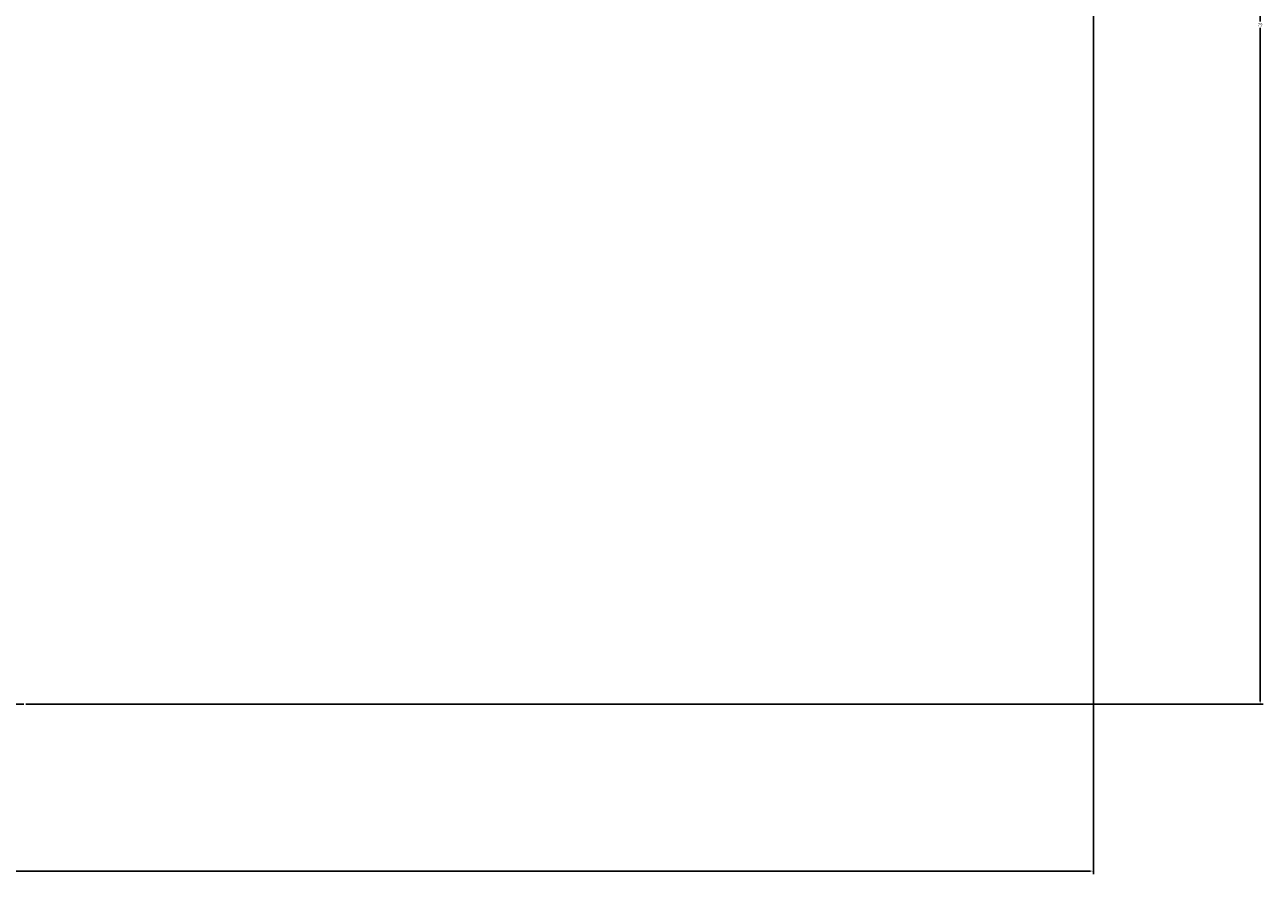
# Model space of a CAD drawing. Units: millimetres. Extents: x -136 to 10, y 158 to 257.
# Tile 4 of 6: x -62 to 10, y 158 to 208. Entities that reach past the tile are written whole.
import ezdxf

# ---------------------------------------------------------------- set-up
doc = ezdxf.new("R2010")
doc.units = ezdxf.units.MM
doc.layers.add('M-DIMS', color=2, linetype='Continuous', lineweight=18)
doc.styles.get("Standard").update_dxf_attribs({"font": 'arial.ttf'})
doc.dimstyles.get("Standard").update_dxf_attribs({"dimtxt": 0.18, "dimasz": 0.18, "dimexe": 0.18, "dimexo": 0.0625, "dimgap": 0.09, "dimtad": 0, "dimtih": 1, "dimtoh": 1, "dimdec": 4, "dimzin": 0, "dimdsep": 46, "dimtxsty": 'Standard', "dimcen": 0.09, "dimadec": 0, "dimazin": 0, "dimtfac": 1, "dimtdec": 4, "dimtofl": 0, "dimtmove": 0, "dimatfit": 3, "dimfxl": 1, "dimtolj": 1, "dimtzin": 0, "dimarcsym": 0})

# ---------------------------------------------------------------- blocks, each defined once
blk = doc.blocks.new('*D1')
at = {"layer": 'Defpoints', "color": 0, "transparency": 16777216}
for p in [(-126, 231.107), (0, 231.107), (0, 158.407)]:
    blk.add_point(p, dxfattribs=at)
at = {"layer": 'M-DIMS', "color": 0, "lineweight": -2, "transparency": 16777216}
for p, q in [((-126, 231.044), (-126, 158.227)), ((0, 231.044), (0, 158.227)), ((-125.82, 158.407), (-63.28, 158.407)), ((-0.18, 158.407), (-62.72, 158.407))]:
    blk.add_line(p, q, dxfattribs=at)
at = {"layer": 'M-DIMS', "color": 0, "transparency": 16777216}
for points in [[(-125.82, 158.437), (-125.82, 158.377), (-126, 158.407)], [(-0.18, 158.437), (-0.18, 158.377), (0, 158.407)]]:
    blk.add_solid(points, dxfattribs=at)
at = {"layer": 'M-DIMS', "color": 0, "transparency": 16777216, "insert": (-63, 158.407), "char_height": 0.18, "attachment_point": 5}
blk.add_mtext('\\A1;126', dxfattribs=at)
blk = doc.blocks.new('*D2')
at = {"layer": 'Defpoints', "color": 0, "transparency": 16777216}
for p in [(0, 247.107), (9.7, 247.107), (-62.158, 168.107)]:
    blk.add_point(p, dxfattribs=at)
at = {"layer": 'M-DIMS', "color": 0, "lineweight": -2, "transparency": 16777216}
for p, q in [((0.062, 247.107), (9.88, 247.107)), ((9.7, 246.927), (9.7, 207.789)), ((9.7, 168.287), (9.7, 207.425)), ((-62.095, 168.107), (9.88, 168.107))]:
    blk.add_line(p, q, dxfattribs=at)
at = {"layer": 'M-DIMS', "color": 0, "transparency": 16777216}
for points in [[(9.67, 246.927), (9.73, 246.927), (9.7, 247.107)], [(9.67, 168.287), (9.73, 168.287), (9.7, 168.107)]]:
    blk.add_solid(points, dxfattribs=at)
at = {"layer": 'M-DIMS', "color": 0, "transparency": 16777216, "insert": (9.7, 207.607), "char_height": 0.18, "attachment_point": 5}
blk.add_mtext('\\A1;79', dxfattribs=at)
blk = doc.blocks.new('*D3')
at = {"layer": 'Defpoints', "color": 0, "transparency": 16777216}
for p in [(-126, 231.107), (-135.7, 168.107), (-62.158, 168.107)]:
    blk.add_point(p, dxfattribs=at)
at = {"layer": 'M-DIMS', "color": 0, "lineweight": -2, "transparency": 16777216}
for p, q in [((-126.062, 231.107), (-135.88, 231.107)), ((-135.7, 230.927), (-135.7, 199.789)), ((-135.7, 168.287), (-135.7, 199.425)), ((-62.22, 168.107), (-135.88, 168.107))]:
    blk.add_line(p, q, dxfattribs=at)
at = {"layer": 'M-DIMS', "color": 0, "transparency": 16777216}
for points in [[(-135.73, 230.927), (-135.67, 230.927), (-135.7, 231.107)], [(-135.73, 168.287), (-135.67, 168.287), (-135.7, 168.107)]]:
    blk.add_solid(points, dxfattribs=at)
at = {"layer": 'M-DIMS', "color": 0, "transparency": 16777216, "insert": (-135.7, 199.607), "char_height": 0.18, "attachment_point": 5}
blk.add_mtext('\\A1;63', dxfattribs=at)

msp = doc.modelspace()

# ---------------------------------------------------------------- dimensions: what is measured, and where the dimension line sits
at = {"layer": 'M-DIMS'}
for base, p1, p2, picture, middle in [((9.7, 247.1068), (-62.158, 168.1068), (0, 247.1068), '*D2', (9.7, 207.6068)), ((-135.7, 168.1068), (-126, 231.1068), (-62.158, 168.1068), '*D3', (-135.7, 199.6068))]:
    dim = msp.add_linear_dim(base=base, p1=p1, p2=p2, angle=90, dimstyle='Standard', override={"dimdec": 0, "dimlfac": 1, "dimrnd": 0, "dimzin": 0, "dimdsep": 46, "dimlunit": 2}, dxfattribs=at)
    dim.commit()
    dim.dimension.update_dxf_attribs({"geometry": picture, "text_midpoint": middle})
dim = msp.add_linear_dim(base=(0, 158.4068), p1=(-126, 231.1068), p2=(0, 231.1068), dimstyle='Standard', override={"dimdec": 0, "dimlfac": 1, "dimrnd": 0, "dimzin": 0, "dimdsep": 46, "dimlunit": 2}, dxfattribs=at)
dim.commit()
dim.dimension.update_dxf_attribs({"geometry": '*D1', "text_midpoint": (-63, 158.4068)})

doc.saveas('drawing.dxf')
